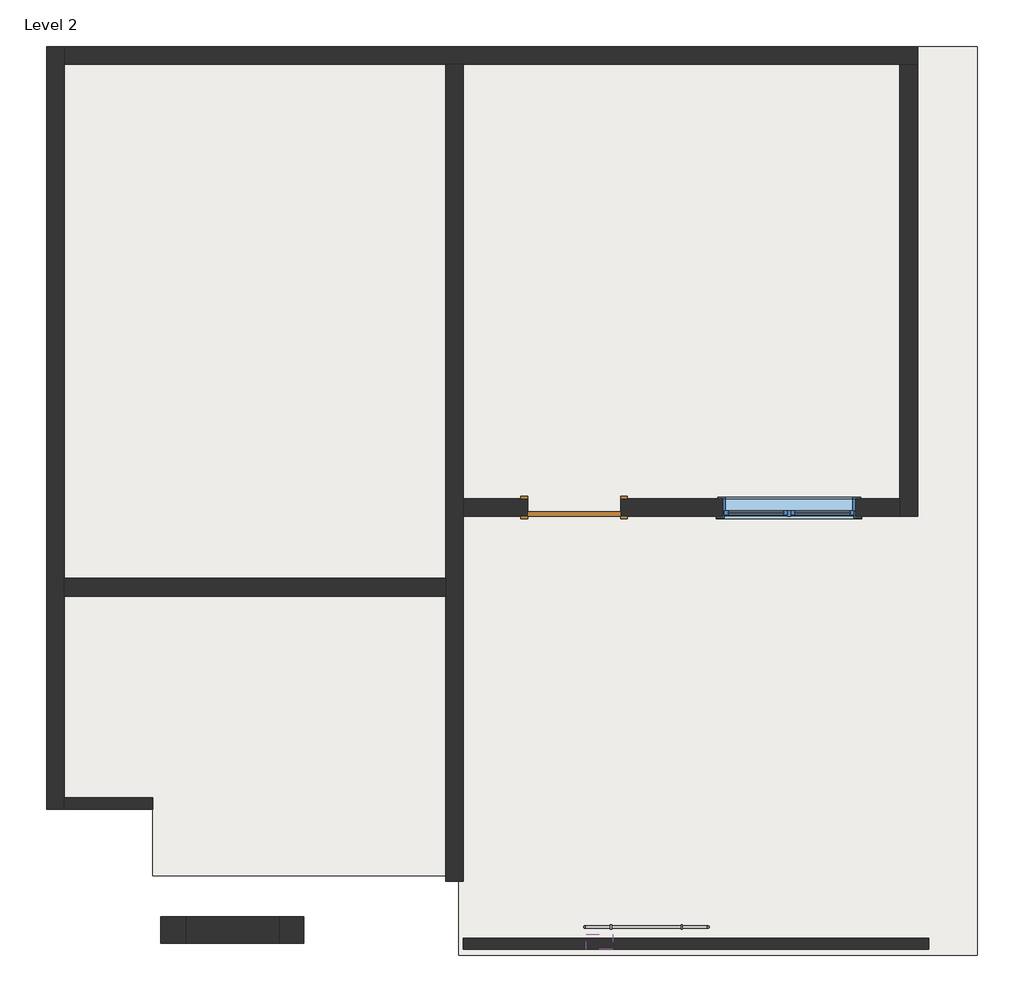
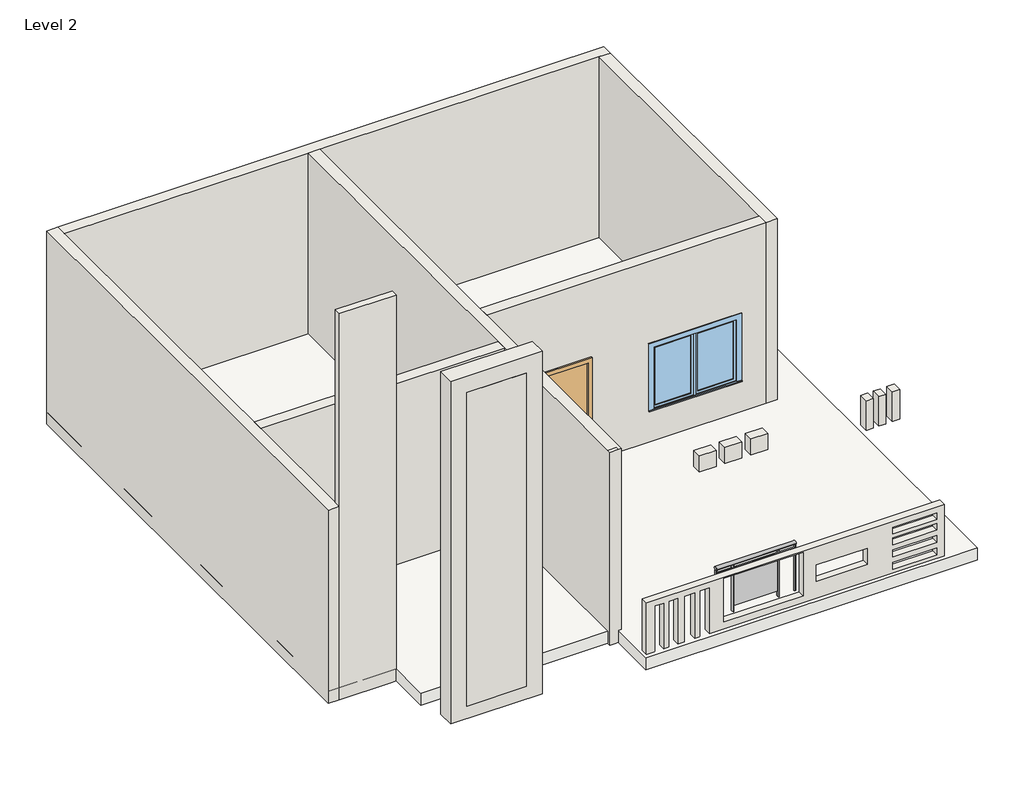
# One storey: 10 walls, 1 door, 1 railing, 1 roof, 1 window.
"""IFC4 building model written with IfcOpenShell, lengths in millimetres."""

from ifc_helpers import new_model, si_unit, point, frame, origin, place, context, project, spatial, polyline, ellipse_curve, trimmed, outline, extrude, faceted_brep, transform, mapped, element, save
from ifc_brep_helpers import plane_surface, extruded_surface, advanced_brep
from components import door_ed2803e5, walls_3_walls_3_7c260857, walls_5_walls_5_e6219bd2, window_03976a38

model = new_model("IFC4")

# Units and contexts
model_context = context("Model", 3, world=origin())
ifc_project = project(units=[si_unit("LENGTHUNIT", "METRE", prefix="MILLI")], contexts=[model_context])

# Site, building, storey
site = spatial("IfcSite", under=ifc_project)
building = spatial("IfcBuilding", under=site)
storey = spatial("IfcBuildingStorey", under=building, Name="Level 2", Elevation=3657.6)

# Door
placement = place(None, origin())
door_shape = door_ed2803e5(model_context)
element("IfcDoor", 1, ObjectType="Door-Single-Panel : 34\" x 80\"", at=placement, inside=storey, context=model_context, shape_type="MappedRepresentation", body=[
    mapped(door_shape, transform((-2660.3936733, 8192.8419215, 3657.6), x_axis=(-1.0, 0.0, 0.0), y_axis=(0.0, -1.0, 0.0), z_axis=(0.0, 0.0, 1.0))),
])

# Railing
element("IfcRailing", 2, ObjectType="Glass Panel - Bottom Fill", at=placement, inside=storey, context=model_context, shape_type="SolidModel", body=[
    advanced_brep(
    [(-2542.411491, 3423.9919215, 4876.8), (-2542.411491, 3347.7919215, 4876.8), (-1120.011491, 3423.9919215, 4876.8), (-1120.011491, 3347.7919215, 4876.8)],
    [
        (0, 1, ellipse_curve(frame((-2542.411491, 3385.8919215, 4876.8), z_axis=(-1.0, 0.0, 0.0), x_axis=(0.0, -1.0, 0.0)), 38.1, 28.575)),
        (1, 0, ellipse_curve(frame((-2542.411491, 3385.8919215, 4876.8), z_axis=(-1.0, 0.0, 0.0), x_axis=(0.0, -1.0, 0.0)), 38.1, 28.575)),
        (2, 3, ellipse_curve(frame((-1120.011491, 3385.8919215, 4876.8), z_axis=(1.0, 0.0, 0.0), x_axis=(0.0, -1.0, 0.0)), 38.1, 28.575)),
        (3, 2, ellipse_curve(frame((-1120.011491, 3385.8919215, 4876.8), z_axis=(1.0, 0.0, 0.0), x_axis=(0.0, -1.0, 0.0)), 38.1, 28.575)),
        (0, 2),
        (3, 1),
    ],
    [
        plane_surface(frame((-2542.411491, 3385.8919215, 4876.8), z_axis=(-1.0, 0.0, 0.0), x_axis=(0.0, 1.0, 0.0))),
        plane_surface(frame((-1120.011491, 3385.8919215, 4876.8), z_axis=(1.0, 0.0, 0.0), x_axis=(0.0, 1.0, 0.0))),
        extruded_surface(trimmed(ellipse_curve(frame((-1120.011491, 3385.8919215, 4876.8), z_axis=(-1.0, 0.0, 0.0), x_axis=(0.0, -1.0, 0.0)), 38.1, 28.575), [point((-1120.011491, 3423.9919215, 4876.8))], [point((-1120.011491, 3347.7919215, 4876.8))], True, "CARTESIAN"), (-1422.3999999999999, 0.0, 0.0), 1422.3999999999999),
        extruded_surface(trimmed(ellipse_curve(frame((-1120.011491, 3385.8919215, 4876.8), z_axis=(-1.0, 0.0, 0.0), x_axis=(0.0, -1.0, 0.0)), 38.1, 28.575), [point((-1120.011491, 3347.7919215, 4876.8))], [point((-1120.011491, 3423.9919215, 4876.8))], True, "CARTESIAN"), (-1422.3999999999999, 0.0, 0.0), 1422.3999999999999),
    ],
    [
        (0, [[1, 2]]),
        (1, [[3, 4]]),
        (2, [[-1, 5, -4, 6]]),
        (3, [[-2, -6, -3, -5]]),
    ],
),
    extrude(outline(polyline([(-2542.411491, 3373.1919215), (-2542.411491, 3398.5919215), (-1120.011491, 3398.5919215), (-1120.011491, 3373.1919215), (-2542.411491, 3373.1919215)])), frame((0.0, 0.0, 4762.5), z_axis=(0.0, 0.0, 1.0), x_axis=(1.0, 0.0, 0.0)), (0.0, 0.0, 1.0), 25.4),
    extrude(outline(polyline([(-2542.411491, 3373.1919215), (-2542.411491, 3398.5919215), (-1120.011491, 3398.5919215), (-1120.011491, 3373.1919215), (-2542.411491, 3373.1919215)])), frame((0.0, 0.0, 4660.9), z_axis=(0.0, 0.0, 1.0), x_axis=(1.0, 0.0, 0.0)), (0.0, 0.0, 1.0), 25.4),
    extrude(outline(polyline([(-1431.161491, 3360.4919215), (-1431.161491, 3411.2919215), (-1418.461491, 3411.2919215), (-1418.461491, 3360.4919215), (-1431.161491, 3360.4919215)])), frame((0.0, 0.0, 3962.4), z_axis=(0.0, 0.0, 1.0), x_axis=(1.0, 0.0, 0.0)), (0.0, 0.0, 1.0), 885.6788223),
    extrude(outline(polyline([(-2237.611491, 3392.4270785), (-1424.811491, 3392.4270785), (-1424.811491, 3386.0770785), (-2237.611491, 3386.0770785), (-2237.611491, 3392.4270785)])), frame((0.0, 0.0, 4064.0), z_axis=(0.0, 0.0, 1.0), x_axis=(1.0, 0.0, 0.0)), (0.0, 0.0, 1.0), 596.9),
    extrude(outline(polyline([(-2243.961491, 3360.4919215), (-2243.961491, 3411.2919215), (-2231.261491, 3411.2919215), (-2231.261491, 3360.4919215), (-2243.961491, 3360.4919215)])), frame((0.0, 0.0, 3962.4), z_axis=(0.0, 0.0, 1.0), x_axis=(1.0, 0.0, 0.0)), (0.0, 0.0, 1.0), 885.6788223),
    extrude(outline(polyline([(-1132.711491, 3376.3669215), (-1132.711491, 3395.4169215), (-1113.661491, 3395.4169215), (-1113.661491, 3376.3669215), (-1132.711491, 3376.3669215)])), frame((0.0, 0.0, 3962.4), z_axis=(0.0, 0.0, 1.0), x_axis=(1.0, 0.0, 0.0)), (0.0, 0.0, 1.0), 885.6788223),
    extrude(outline(polyline([(-2548.761491, 3376.3669215), (-2548.761491, 3395.4169215), (-2529.711491, 3395.4169215), (-2529.711491, 3376.3669215), (-2548.761491, 3376.3669215)])), frame((0.0, 0.0, 3962.4), z_axis=(0.0, 0.0, 1.0), x_axis=(1.0, 0.0, 0.0)), (0.0, 0.0, 1.0), 885.6788223),
])

# Roof
element("IfcRoof", 3, ObjectType="Generic - 9\"", at=placement, inside=storey, context=model_context, shape_type="SweptSolid", body=[
    extrude(outline(polyline([(-8705.5936733, 13476.0419215), (1962.4063267, 13476.0419215), (1962.4063267, 3722.4419215), (1962.4063267, 3062.0419215), (-3981.1936733, 3062.0419215), (-3981.1936733, 3976.4419215), (-7486.3936733, 3976.4419215), (-7486.3936733, 4738.4419215), (-8705.5936733, 4738.4419215), (-8705.5936733, 13476.0419215)])), frame((0.0, 0.0, 3657.6), z_axis=(0.0, 0.0, 1.0), x_axis=(1.0, 0.0, 0.0)), (0.0, 0.0, 1.0), 228.6),
])

# Walls
element("IfcWall", 4, ObjectType="Generic - 5\"", at=placement, inside=storey, context=model_context, shape_type="Brep", body=[
    faceted_brep([(-7486.3936733, 4865.4419215, 3657.6), (-8502.3936733, 4865.4419215, 3657.6), (-8502.3936733, 4865.4419215, 10972.8), (-7486.3936733, 4865.4419215, 10972.8), (-7486.3936733, 4738.4419215, 3657.6), (-7486.3936733, 4738.4419215, 10972.8), (-8502.3936733, 4738.4419215, 10972.8), (-8502.3936733, 4738.4419215, 7315.2), (-8502.3936733, 4738.4419215, 3657.6), (-7613.3936733, 4738.4419215, 3657.6)], [[[0, 1, 2, 3]], [[4, 5, 6, 7, 8, 9]], [[1, 0, 4, 9, 8]], [[3, 2, 6, 5]], [[0, 3, 5, 4]], [[1, 8, 7, 6, 2]]]),
])
element("IfcWall", 5, ObjectType="Generic - 5\"", at=placement, inside=storey, context=model_context, shape_type="SweptSolid", body=[
    extrude(outline(polyline([(3657.6, -3930.3936733), (3657.6, 1403.6063267), (4867.5410909, 1403.6063267), (4867.5410909, -3930.3936733), (3657.6, -3930.3936733)]), holes=[polyline([(4750.9410475, -3620.6215053), (3760.3410475, -3620.6215053), (3760.3410475, -3773.0215053), (4750.9410475, -3773.0215053), (4750.9410475, -3620.6215053)]), polyline([(4750.9410475, -3364.9892798), (3760.3410475, -3364.9892798), (3760.3410475, -3521.6717373), (4750.9410475, -3521.6717373), (4750.9410475, -3364.9892798)]), polyline([(4750.9410475, -3065.4492875), (3760.3410475, -3065.4492875), (3760.3410475, -3240.5649753), (4750.9410475, -3240.5649753), (4750.9410475, -3065.4492875)]), polyline([(4750.9410475, -2802.7757558), (3760.3410475, -2802.7757558), (3760.3410475, -2968.6748284), (4750.9410475, -2968.6748284), (4750.9410475, -2802.7757558)]), polyline([(4514.0665497, 28.6801951), (4209.2665497, 28.6801951), (4209.2665497, -885.7198049), (4514.0665497, -885.7198049), (4514.0665497, 28.6801951)]), polyline([(4750.9410475, 489.2063267), (4750.9410475, 1276.6063267), (4623.9410475, 1276.6063267), (4623.9410475, 489.2063267), (4750.9410475, 489.2063267)]), polyline([(4544.8002436, 489.2063267), (4544.8002436, 1276.6063267), (4420.3759391, 1276.6063267), (4420.3759391, 489.2063267), (4544.8002436, 489.2063267)]), polyline([(4323.5665497, 489.2063267), (4323.5665497, 1276.6063267), (4185.9690226, 1276.6063267), (4185.9690226, 489.2063267), (4323.5665497, 489.2063267)]), polyline([(4083.523692, 489.2063267), (4083.523692, 1276.6063267), (3952.7830254, 1276.6063267), (3952.7830254, 489.2063267), (4083.523692, 489.2063267)]), polyline([(4839.8410475, -1120.011491), (4014.3410475, -1120.011491), (4014.3410475, -2542.411491), (4839.8410475, -2542.411491), (4839.8410475, -1120.011491)])]), frame((0.0, 3131.8919215, 0.0), z_axis=(0.0, 1.0, 0.0), x_axis=(0.0, 0.0, 1.0)), (0.0, 0.0, 1.0), 127.0),
])
element("IfcWall", 6, ObjectType="Generic - 8\"", at=placement, inside=storey, context=model_context, shape_type="Brep", body=[
    faceted_brep([(-8502.3936733, 4738.4419215, 3657.6), (-8502.3936733, 4865.4419215, 3657.6), (-8502.3936733, 7176.8419215, 3657.6), (-8502.3936733, 7380.0419215, 3657.6), (-8502.3936733, 13272.8419215, 3657.6), (-8502.3936733, 13476.0419215, 3657.6), (-8502.3936733, 13476.0419215, 7315.2), (-8502.3936733, 13272.8419215, 7315.2), (-8502.3936733, 8091.2419215, 7315.2), (-8502.3936733, 7380.0419215, 7315.2), (-8502.3936733, 7176.8419215, 7315.2), (-8502.3936733, 4738.4419215, 7315.2), (-8705.5936733, 4738.4419215, 3657.6), (-8705.5936733, 4738.4419215, 7315.2), (-8705.5936733, 8091.2419215, 7315.2), (-8705.5936733, 13476.0419215, 7315.2), (-8705.5936733, 13476.0419215, 3657.6)], [[[0, 1, 2, 3, 4, 5, 6, 7, 8, 9, 10, 11]], [[12, 13, 14, 15, 16]], [[5, 4, 3, 2, 1, 0, 12, 16]], [[6, 5, 16, 15]], [[0, 11, 13, 12]], [[11, 10, 9, 8, 7, 6, 15, 14, 13]]]),
])
element("IfcWall", 7, ObjectType="Generic - 8\"", at=placement, inside=storey, context=model_context, shape_type="SweptSolid", body=[
    extrude(outline(polyline([(-4133.5936733, 7176.8419215), (-8502.3936733, 7176.8419215), (-8502.3936733, 7380.0419215), (-4133.5936733, 7380.0419215), (-4133.5936733, 7176.8419215)])), frame((0.0, 0.0, 3657.6), z_axis=(0.0, 0.0, 1.0), x_axis=(1.0, 0.0, 0.0)), (0.0, 0.0, 1.0), 3657.6),
])
element("IfcWall", 8, ObjectType="Generic - 8\"", at=placement, inside=storey, context=model_context, shape_type="Brep", body=[
    faceted_brep([(-4133.5936733, 13272.8419215, 3657.6), (-4133.5936733, 7380.0419215, 3657.6), (-4133.5936733, 7176.8419215, 3657.6), (-4133.5936733, 4039.9419215, 3657.6), (-4133.5936733, 3912.9419215, 3657.6), (-4133.5936733, 3912.9419215, 7315.2), (-4133.5936733, 3976.4419215, 7315.2), (-4133.5936733, 4039.9419215, 7315.2), (-4133.5936733, 7176.8419215, 7315.2), (-4133.5936733, 7380.0419215, 7315.2), (-4133.5936733, 13272.8419215, 7315.2), (-3930.3936733, 13272.8419215, 3657.6), (-3930.3936733, 13272.8419215, 7315.2), (-3930.3936733, 8294.4419215, 7315.2), (-3930.3936733, 8091.2419215, 7315.2), (-3930.3936733, 3912.9419215, 7315.2), (-3930.3936733, 3912.9419215, 3657.6), (-3930.3936733, 8091.2419215, 3657.6), (-3930.3936733, 8294.4419215, 3657.6), (-3955.7936733, 3912.9419215, 3657.6), (-4082.7936733, 3912.9419215, 3657.6), (-3981.1936733, 13272.8419215, 7315.2), (-3981.1936733, 3912.9419215, 7315.2), (-3981.1936733, 3976.4419215, 7315.2), (-3955.7936733, 3912.9419215, 7315.2)], [[[0, 1, 2, 3, 4, 5, 6, 7, 8, 9, 10]], [[11, 12, 13, 14, 15, 16, 17, 18]], [[4, 3, 2, 1, 0, 11, 18, 17, 16, 19, 20]], [[0, 10, 21, 12, 11]], [[6, 5, 22, 23]], [[22, 24, 15, 14, 13, 12, 21, 10, 9, 8, 7, 6, 23]], [[4, 20, 19, 16, 15, 24, 22, 5]]]),
])
element("IfcWall", 9, ObjectType="Generic - 8\"", at=placement, inside=storey, context=model_context, shape_type="Brep", body=[
    faceted_brep([(-8502.3936733, 13272.8419215, 3657.6), (-4133.5936733, 13272.8419215, 3657.6), (-3930.3936733, 13272.8419215, 3657.6), (1073.4063267, 13272.8419215, 3657.6), (1276.6063267, 13272.8419215, 3657.6), (1276.6063267, 13272.8419215, 7315.2), (1073.4063267, 13272.8419215, 7315.2), (-3930.3936733, 13272.8419215, 7315.2), (-4133.5936733, 13272.8419215, 7315.2), (-8502.3936733, 13272.8419215, 7315.2), (-8502.3936733, 13476.0419215, 3657.6), (-8502.3936733, 13476.0419215, 7315.2), (1276.6063267, 13476.0419215, 7315.2), (1276.6063267, 13476.0419215, 3657.6)], [[[0, 1, 2, 3, 4, 5, 6, 7, 8, 9]], [[10, 11, 12, 13]], [[4, 3, 2, 1, 0, 10, 13]], [[0, 9, 11, 10]], [[5, 4, 13, 12]], [[9, 8, 7, 6, 5, 12, 11]]]),
])
element("IfcWall", 10, ObjectType="Generic - 8\"", at=placement, inside=storey, context=model_context, shape_type="Brep", body=[
    faceted_brep([(1073.4063267, 13272.8419215, 3657.6), (1073.4063267, 8294.4419215, 3657.6), (1073.4063267, 8091.2419215, 3657.6), (1073.4063267, 8091.2419215, 7315.2), (1073.4063267, 8294.4419215, 7315.2), (1073.4063267, 13272.8419215, 7315.2), (1276.6063267, 13272.8419215, 3657.6), (1276.6063267, 13272.8419215, 7315.2), (1276.6063267, 8091.2419215, 7315.2), (1276.6063267, 8091.2419215, 3657.6)], [[[0, 1, 2, 3, 4, 5]], [[6, 7, 8, 9]], [[2, 1, 0, 6, 9]], [[0, 5, 7, 6]], [[3, 2, 9, 8]], [[5, 4, 3, 8, 7]]]),
])
element("IfcWall", 11, ObjectType="Generic - 8\"", at=placement, inside=storey, context=model_context, shape_type="SweptSolid", body=[
    extrude(outline(polyline([(3657.6, -3930.3936733), (3657.6, -3193.7936733), (5791.2, -3193.7936733), (5791.2, -2126.9936733), (3657.6, -2126.9936733), (3657.6, 1073.4063267), (7315.2, 1073.4063267), (7315.2, -3930.3936733), (3657.6, -3930.3936733)]), holes=[polyline([(5689.6, -958.5936733), (5689.6, 565.4063267), (4470.4, 565.4063267), (4470.4, -958.5936733), (5689.6, -958.5936733)])]), frame((0.0, 8091.2419215, 0.0), z_axis=(0.0, 1.0, 0.0), x_axis=(0.0, 0.0, 1.0)), (0.0, 0.0, 1.0), 203.2),
])
walls_3_walls_3_shape = walls_3_walls_3_7c260857(model_context)
element("IfcWall", 12, ObjectType="Walls 3 : Walls 3", at=placement, inside=storey, context=model_context, shape_type="MappedRepresentation", body=[
    mapped(walls_3_walls_3_shape, transform((-152.4, 0.0, 0.0), x_axis=(1.0, 0.0, 0.0), y_axis=(0.0, 1.0, 0.0), z_axis=(0.0, 0.0, 1.0))),
])
walls_5_walls_5_shape = walls_5_walls_5_e6219bd2(model_context)
element("IfcWall", 13, ObjectType="Walls 5 : Walls 5", at=placement, inside=storey, context=model_context, shape_type="MappedRepresentation", body=[
    mapped(walls_5_walls_5_shape, transform((0.0, 0.0, 0.0), x_axis=(1.0, 0.0, 0.0), y_axis=(0.0, 1.0, 0.0), z_axis=(0.0, 0.0, 1.0))),
])

# Window
window_shape = window_03976a38(model_context)
element("IfcWindow", 14, ObjectType="Casement Dbl with Trim : 48\" x 48\"", at=placement, inside=storey, context=model_context, shape_type="MappedRepresentation", body=[
    mapped(window_shape, transform((-196.5936733, 8211.8919215, 3556.0), x_axis=(-1.0, 0.0, 0.0), y_axis=(0.0, -1.0, 0.0), z_axis=(0.0, 0.0, 1.0))),
])

save(model, "model.ifc")

# Revit data of these elements
# Type "Door-Single-Panel : 34\" x 80\""
#   Type Mark = "8"
#   Construction Type Id = "DOOR"
#   Assembly Code = "C1020300"
#   Analytic Construction = "Wooden"
#   Thickness = 0' - 2"
#   Thermal Resistance (R) = 2.5876 (h·ft²·°F)/BTU
#   Swing Angle [instance default] = 90.00°
#   Heat Transfer Coefficient (U) = 0.3865 BTU/(h·ft²·°F)
#   Height = 7' - 0"
#   Trim Projection Ext = 0' - 1"
#   Trim Projection Int = 0' - 1"
#   Trim Width = 0' - 3"
#   Width = 3' - 6"
#   Define Thermal Properties by = 1
#   Panel Material = Wood - Birch - Solid Stained Light Low Gloss
#   Trim Material = Paint - Sienna
#   Visual Light Transmittance = 0
#   Solar Heat Gain Coefficient = 0
#   Function = (empty or 0)
#   Wall Closure = (empty or 0)
# Type "Glass Panel - Bottom Fill"
#   Assembly Code = "C2010400"
#   built-in parameter 1008612 = 0.0416667 (stored number, unit not read)
#   built-in parameter 1008611 = 0.0416667 (stored number, unit not read)
#   built-in parameter 1008609 = 0.333333 (stored number, unit not read)
#   built-in parameter 1008604 = 0.166667 (stored number, unit not read)
#   built-in parameter 1008603 = 0.166667 (stored number, unit not read)
#   Railing Height = 3' - 0"
#   built-in parameter 1008630 = 2
#   built-in parameter 1008610 = 2
#   built-in parameter 1008618 = Baluster - Square : 3/4"
# Type "Generic - 9\""
#   Assembly Code = "B1020"
#   Layers, outside or top first: 0' - 9" no material (function 1)
# Type "Generic - 5\""
#   Assembly Code = "B2010"
#   Layers, outside or top first: 0' - 5" no material (function 1)
# Type "Generic - 8\""
#   Assembly Code = "B2010"
#   Layers, outside or top first: 0' - 8" no material (function 1)
# Type "Casement Dbl with Trim : 48\" x 48\""
#   Type Mark = "10"
#   Construction Type Id = "GSP4R"
#   Assembly Code = "B2020100"
#   Analytic Construction = "1/8 in Pilkington single glazing"
#   Visual Light Transmittance = 0.9
#   Solar Heat Gain Coefficient = 0.78
#   Heat Transfer Coefficient (U) = 0.6496 BTU/(h·ft²·°F)
#   Height = 4' - 0"
#   Default Sill Height = 3' - 0"
#   Trim Projection - Ext. = 0' - 0 1/2"
#   Trim Projection - Int. = 0' - 0 3/4"
#   Trim Width - Exterior = 0' - 3 1/2"
#   Trim Width - Interior = 0' - 3 1/2"
#   Width = 5' - 0"
#   Window Inset = 0' - 0 3/4"
#   Define Thermal Properties by = 1
#   Glass Pane Material = Glass
#   Sash Material = Sash
#   Trim Exterior Material = Trim
#   Trim Interior Material = Trim
#   Wall Closure = (empty or 0)
# Element 1 (IfcDoor, "Door-Single-Panel : 34\" x 80\"")
#   Swing Angle = 90.00°
#   Phase Created = New Construction
#   Materials on its faces: "Paint - Sienna", "Wood - Birch - Solid Stained Light Low Gloss"
# Element 2 (IfcRailing, "Glass Panel - Bottom Fill")
#   built-in parameter 1008621 = 1 (stored number, unit not read)
#   Phase Created = New Construction
#   Materials on its faces: "Glass"
# Element 3 (IfcRoof, "Generic - 9\"")
#   built-in parameter 1001705 = 12.75 (stored number, unit not read)
#   built-in parameter 1001710 = 33615
#   Phase Created = New Construction
#   Materials on its faces: "Default Roof"
# Element 4 (IfcWall, "Generic - 5\"")
#   Top Offset = 12' - 0"
#   Base Offset = 0' - 0"
#   wall height = 24' - 0"
#   Phase Created = New Construction
#   Base Constraint = Level 2
#   Top Constraint = Level 3
#   Materials on its faces: "Default Wall"
# Element 5 (IfcWall, "Generic - 5\"")
#   Top Offset = -8' - 0.36452"
#   Base Offset = 0' - 0"
#   wall height = 3' - 11.63548"
#   Phase Created = New Construction
#   Base Constraint = Level 2
#   Top Constraint = Level 3
#   Materials on its faces: "Default Wall"
# Elements 6, 7, 8, 9, 10, 11 (IfcWall, "Generic - 8\"")
#   Top Offset = 0' - 0"
#   Base Offset = 0' - 0"
#   Unconnected Height = 12' - 0"
#   wall height = 12' - 0"
#   Phase Created = New Construction
#   Base Constraint = Level 2
#   Materials on its faces: "Default Wall"
# Element 12 (IfcWall, "Walls 3 : Walls 3")
#   Phase Created = New Construction
#   Materials on its faces: "Default Wall"
# Element 13 (IfcWall, "Walls 5 : Walls 5")
#   Phase Created = New Construction
#   Materials on its faces: "Default Wall"
# Element 14 (IfcWindow, "Casement Dbl with Trim : 48\" x 48\"")
#   Mark = "1"
#   Phase Created = New Construction
#   Materials on its faces: "Sash", "Trim", "Glass"
# Materials
#   "Wood - Birch - Solid Stained Light Low Gloss": class "Wood", colour RGB 210 159 95, transparency 0, Cost = 0
#   "Paint - Sienna": colour RGB 118 70 51, transparency 0, Cost = 0
#   "Glass": class "Glass", colour RGB 0 128 192, transparency 0.75, Description = "Soda Lime Glass", Cost = 0
#   "Sash": class "Wood", colour RGB 224 178 126, transparency 0
#   "Trim": class "Wood", colour RGB 224 178 126, transparency 0
#   "Default Roof": colour RGB 88 101 114, transparency 0
#   "Default Wall": colour RGB 128 128 128, transparency 0
